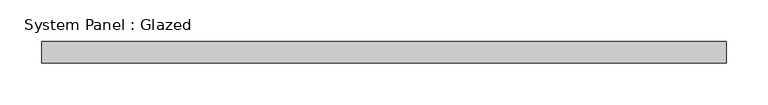
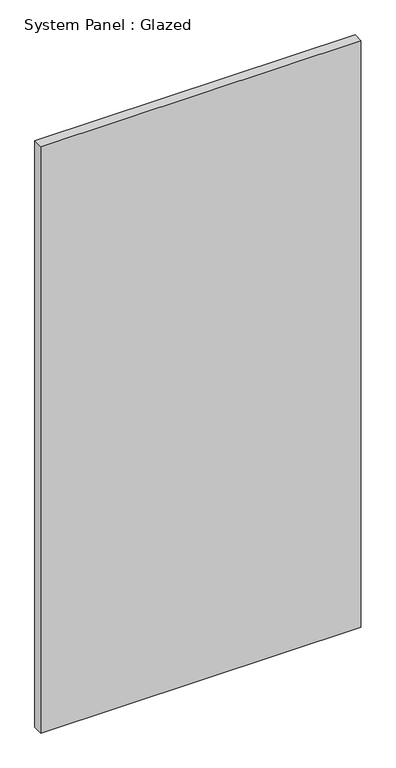
"""IFC4 building model written with IfcOpenShell, lengths in millimetres: plate geometry, System Panel : Glazed."""

from ifc_helpers import new_model, si_unit, origin, origin_with_axes, place, context, project, spatial, polyline, outline, extrude, source, transform, mapped, element, save


def system_panel_glazed_0e71bc1b(model_context):
    return source(origin(), model_context, "Body", "SweptSolid", [
        extrude(outline(polyline([(407.9875, -44.45), (-407.9875, -44.45), (-407.9875, -19.05), (407.9875, -19.05), (407.9875, -44.45)])), origin_with_axes(), (0.0, 0.0, 1.0), 1580.486558),
    ])


if __name__ == "__main__":
    model = new_model("IFC4")
    model_context = context("Model", 3, world=origin())
    ifc_project = project(units=[si_unit("LENGTHUNIT", "METRE", prefix="MILLI")], contexts=[model_context])
    site = spatial("IfcSite", under=ifc_project)
    building = spatial("IfcBuilding", under=site)
    placement = place(None, origin())
    system_panel_glazed_shape = system_panel_glazed_0e71bc1b(model_context)
    element("IfcPlate", 1, ObjectType="System Panel : Glazed", at=placement, inside=building, context=model_context, shape_type="MappedRepresentation", body=[
        mapped(system_panel_glazed_shape, transform((0.0, 0.0, 0.0), x_axis=(1.0, 0.0, 0.0), y_axis=(0.0, 1.0, 0.0), z_axis=(0.0, 0.0, 1.0))),
    ])
    save(model, "model.ifc")

# Revit data of these elements
# Type "System Panel : Glazed"
#   Construction Type Id = "GSP4R"
#   Analytic Construction = "1/8 in Pilkington single glazing"
#   Visual Light Transmittance = 0.9
#   Solar Heat Gain Coefficient = 0.86
#   Heat Transfer Coefficient (U) = 1.18115 BTU/(h·ft²·°F)
#   Define Thermal Properties by = 1
# Element 1 (IfcPlate, "System Panel : Glazed")
#   Materials on its faces: "Glass"
# Materials
#   "Glass": class "Glass", colour RGB 0 128 192, transparency 0.75, Description = "Soda Lime Glass", Cost = 0
